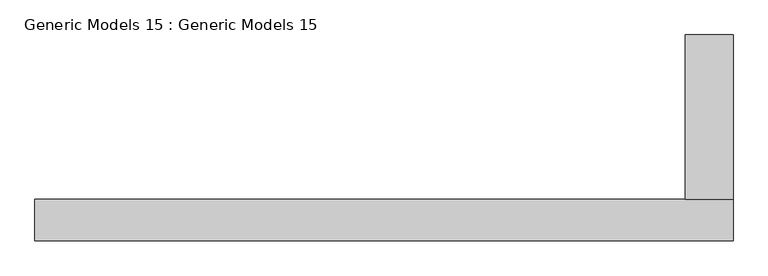
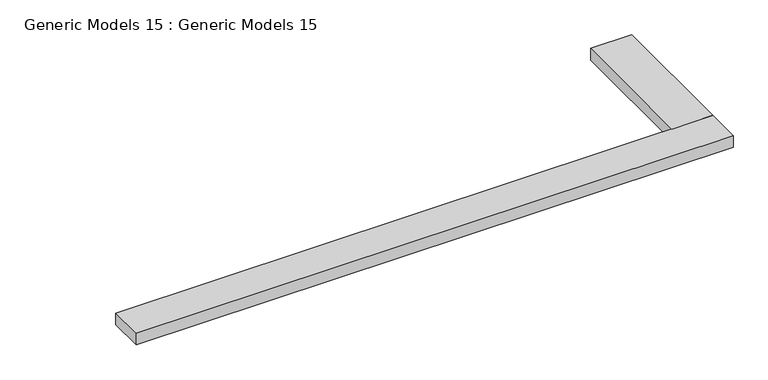
"""IFC4 building model written with IfcOpenShell, lengths in millimetres: proxy geometry, Generic Models 15 : Generic Models 15."""

from ifc_helpers import new_model, si_unit, frame, origin, place, context, project, spatial, polyline, outline, extrude, source, transform, mapped, element, save


def generic_models_15_generic_models_15_609883ec(model_context):
    return source(origin(), model_context, "Body", "SweptSolid", [
        extrude(outline(polyline([(-5165.9536806, -3719.1273102), (-4654.7786806, -3719.1273102), (-4654.7786806, -5471.7273102), (-5165.9536806, -5471.7273102), (-5165.9536806, -3719.1273102)])), frame((0.0, 0.0, 3048.0), z_axis=(0.0, 0.0, 1.0), x_axis=(1.0, 0.0, 0.0)), (0.0, 0.0, 1.0), 152.4),
        extrude(outline(polyline([(-4654.7786806, -5914.3601786), (-12100.1536806, -5914.3601786), (-12100.1536806, -5471.7273102), (-4654.7786806, -5471.7273102), (-4654.7786806, -5914.3601786)])), frame((0.0, 0.0, 3048.0), z_axis=(0.0, 0.0, 1.0), x_axis=(1.0, 0.0, 0.0)), (0.0, 0.0, 1.0), 152.4),
    ])


if __name__ == "__main__":
    model = new_model("IFC4")
    model_context = context("Model", 3, world=origin())
    ifc_project = project(units=[si_unit("LENGTHUNIT", "METRE", prefix="MILLI")], contexts=[model_context])
    site = spatial("IfcSite", under=ifc_project)
    building = spatial("IfcBuilding", under=site)
    placement = place(None, origin())
    generic_models_15_generic_models_15_shape = generic_models_15_generic_models_15_609883ec(model_context)
    element("IfcBuildingElementProxy", 1, Name="Generic Models 15 : Generic Models 15", ObjectType="Generic Models 15 : Generic Models 15", at=placement, inside=building, context=model_context, shape_type="MappedRepresentation", body=[
        mapped(generic_models_15_generic_models_15_shape, transform((0.0, 0.0, 0.0), x_axis=(1.0, 0.0, 0.0), y_axis=(0.0, 1.0, 0.0), z_axis=(0.0, 0.0, 1.0))),
    ])
    save(model, "model.ifc")

# Revit data of these elements
# Element 1 (IfcBuildingElementProxy, "Generic Models 15 : Generic Models 15")
#   Materials on its faces: "exterior wall", "wall"
# Materials
#   "exterior wall": class "Generic", colour RGB 215 217 121, transparency 0, Cost = 0
#   "wall": class "Generic", colour RGB 127 127 127, transparency 0, Cost = 0
